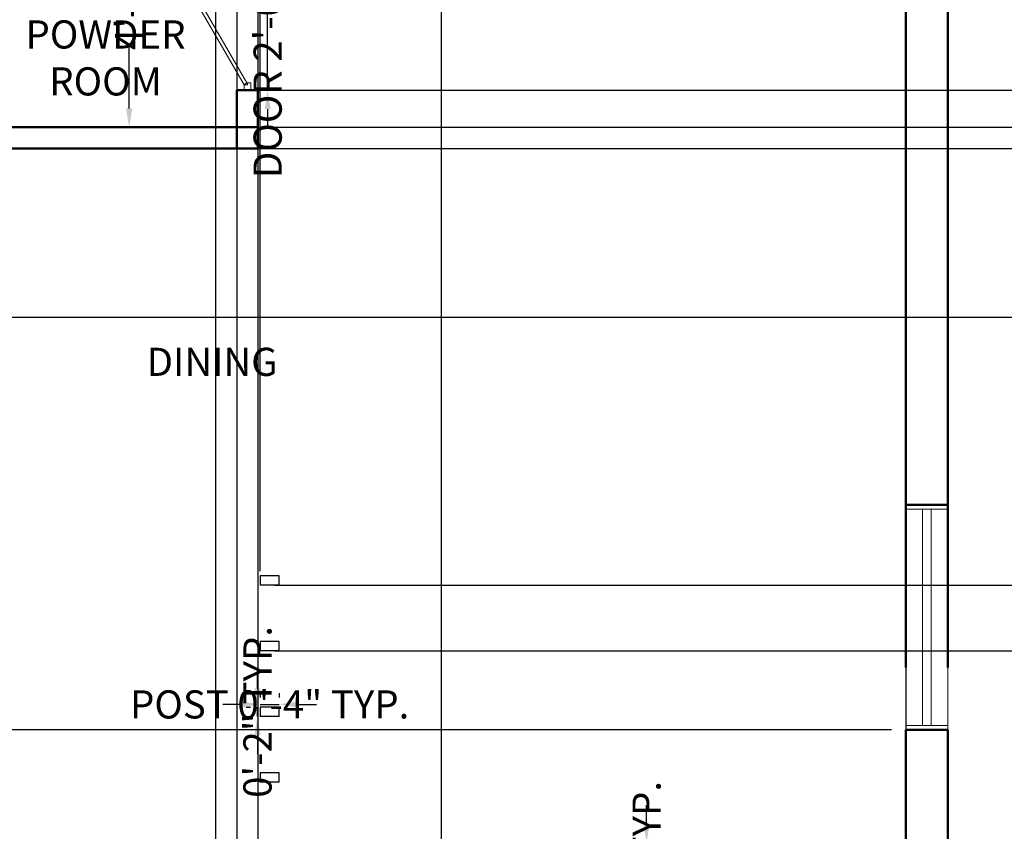
# Model space of a CAD drawing. Units: inches. Extents: x 6704 to 7574, y 11759 to 12617.
# Tile 5 of 8: x 7071 to 7281, y 12195 to 12368. Entities that reach past the tile are written whole.
import ezdxf

# ---------------------------------------------------------------- set-up
doc = ezdxf.new("R2010")
doc.units = ezdxf.units.IN
doc.header["$MEASUREMENT"] = 0
for name, color, linetype, lineweight in [('A-AREA-IDEN', 7, 'Continuous', 18), ('A-DOOR', 4, 'Continuous', 20), ('A-FLOR-SCRN', 7, 'Continuous', 25), ('WALL', 7, 'Continuous', 50), ('WINDOW', 2, 'Continuous', 20), ('YQ_DIM', 3, 'Continuous', 18)]:
    doc.layers.add(name, color=color, linetype=linetype, lineweight=lineweight)
doc.styles.get("Standard").update_dxf_attribs({"font": 'arial.ttf'})
doc.styles.add('YQ_DIM', font='SUPEROS.SHX', dxfattribs={"width": 0.8, "bigfont": 'HZDX.SHX'})
doc.dimstyles.new('yqi0', dxfattribs={"dimscale": 0, "dimtxt": 6, "dimasz": 4, "dimexe": 1.5, "dimexo": 3, "dimgap": 0.5, "dimtad": 0, "dimdsep": 46, "dimlunit": 4, "dimtxsty": 'Standard', "dimcen": 0, "dimclrd": 256, "dimclre": 256, "dimclrt": 7, "dimadec": 1, "dimazin": 2, "dimtfac": 1, "dimtix": 1, "dimtmove": 2, "dimatfit": 2, "dimfxl": 1, "dimtolj": 1, "dimtzin": 0, "dimarcsym": 0})

# ---------------------------------------------------------------- blocks, each defined once
blk = doc.blocks.new('*D5')
at = {"layer": 'Defpoints', "color": 0, "transparency": 16777216}
for p in [(7090.57, 12400.26), (7090.57, 12344.76), (7094.64, 12344.76)]:
    blk.add_point(p, dxfattribs=at)
at = {"layer": 'YQ_DIM', "color": 0, "lineweight": -2, "transparency": 16777216}
for p, q in [((7093.57, 12400.26), (7096.14, 12400.26)), ((7094.64, 12396.26), (7094.64, 12383.29)), ((7094.64, 12348.76), (7094.64, 12361.72)), ((7093.57, 12344.76), (7096.14, 12344.76))]:
    blk.add_line(p, q, dxfattribs=at)
at = {"layer": 'YQ_DIM', "color": 0, "transparency": 16777216}
for points in [[(7093.97, 12396.26), (7095.31, 12396.26), (7094.64, 12400.26)], [(7093.97, 12348.76), (7095.31, 12348.76), (7094.64, 12344.76)]]:
    blk.add_solid(points, dxfattribs=at)
at = {"layer": 'YQ_DIM', "color": 0, "transparency": 16777216, "insert": (7094.64, 12372.51), "char_height": 6, "attachment_point": 5, "rotation": 90}
blk.add_mtext('\\A1;4\'-7{\\H1x;\\S1/2;}"', dxfattribs=at)
blk = doc.blocks.new('WD_00_X1')
for p, q in [((-0.5, 0.5), (0.5, 0.5)), ((-0.48, 0.5), (-0.48, -0.5)), ((0.48, 0.5), (0.48, -0.5)), ((0.48, 0.1), (-0.48, 0.1)), ((0.48, -0.1), (-0.48, -0.1)), ((-0.5, -0.5), (0.5, -0.5))]:
    blk.add_line(p, q)
blk = doc.blocks.new('DR_CDR1')
for p, q in [((0.3294, 0.48), (-0.45, 0.03)), ((-0.435, 0.004), (0.3444, 0.454)), ((0.3294, 0.48), (0.3444, 0.454)), ((-0.45, 0.03), (-0.5, 0.03)), ((-0.435, 0.004), (-0.45, 0.03)), ((-0.45, 0.03), (-0.45, 0)), ((-0.45, 0), (-0.435, 0)), ((-0.435, 0), (-0.435, -0.03)), ((0.435, 0), (0.45, 0)), ((0.435, 0), (0.435, -0.03)), ((0.45, 0.03), (0.45, 0)), ((0.5, 0.03), (0.45, 0.03)), ((-0.435, -0.03), (-0.5, -0.03)), ((0.435, -0.03), (0.5, -0.03))]:
    blk.add_line(p, q)
blk.add_lwpolyline([(0.3444, 0.454, -0.121959), (0.45, 0.03)], format="xyb")
blk = doc.blocks.new('DIVIDER-POST-2X4')
for p, q in [((4, 2), (0, 2)), ((0, 2), (0, 0)), ((4, 0), (4, 2)), ((4, 0), (0, 0))]:
    blk.add_line(p, q)
blk = doc.blocks.new('*D26')
at = {"layer": 'Defpoints', "color": 0, "transparency": 16777216}
for p in [(7204.87, 12192.3), (7212.07, 12192.3), (7212.07, 12167.82)]:
    blk.add_point(p, dxfattribs=at)
at = {"layer": 'YQ_DIM', "lineweight": -2, "transparency": 16777216}
for p, q in [((7204.87, 12196.3), (7204.87, 12200.3)), ((7209.07, 12192.3), (7203.37, 12192.3)), ((7204.87, 12167.82), (7204.87, 12192.3)), ((7209.07, 12167.82), (7203.37, 12167.82)), ((7204.87, 12163.82), (7204.87, 12159.82))]:
    blk.add_line(p, q, dxfattribs=at)
at = {"layer": 'YQ_DIM', "transparency": 16777216}
for points in [[(7204.21, 12196.3), (7205.54, 12196.3), (7204.87, 12192.3)], [(7204.21, 12163.82), (7205.54, 12163.82), (7204.87, 12167.82)]]:
    blk.add_solid(points, dxfattribs=at)
at = {"layer": 'YQ_DIM', "color": 7, "transparency": 16777216, "insert": (7204.87, 12180.06), "char_height": 6, "attachment_point": 5, "rotation": 90}
blk.add_mtext('\\A1;2\'-0 1/2" TYP.', dxfattribs=at)
blk = doc.blocks.new('*D29')
at = {"layer": 'Defpoints', "color": 0, "transparency": 16777216}
for p in [(7120.54, 12376.63), (7124.14, 12376.63), (7120.54, 12352.63)]:
    blk.add_point(p, dxfattribs=at)
at = {"layer": 'YQ_DIM', "lineweight": -2, "transparency": 16777216}
for p, q in [((7124.14, 12380.63), (7124.14, 12384.63)), ((7123.54, 12376.63), (7125.64, 12376.63)), ((7124.14, 12352.63), (7124.14, 12376.63)), ((7123.54, 12352.63), (7125.64, 12352.63)), ((7124.14, 12348.63), (7124.14, 12344.63))]:
    blk.add_line(p, q, dxfattribs=at)
at = {"layer": 'YQ_DIM', "transparency": 16777216}
for points in [[(7123.48, 12380.63), (7124.81, 12380.63), (7124.14, 12376.63)], [(7123.48, 12348.63), (7124.81, 12348.63), (7124.14, 12352.63)]]:
    blk.add_solid(points, dxfattribs=at)
at = {"layer": 'YQ_DIM', "color": 7, "transparency": 16777216, "insert": (7124.14, 12364.63), "char_height": 6, "attachment_point": 5, "rotation": 90}
blk.add_mtext('\\A1;DOOR 2\'-0" TYP.', dxfattribs=at)
blk = doc.blocks.new('*D51')
at = {"layer": 'Defpoints', "color": 0, "transparency": 16777216}
for p in [(7122.57, 12221.15), (7126.57, 12221.75), (7126.57, 12221.15)]:
    blk.add_point(p, dxfattribs=at)
at = {"layer": 'YQ_DIM', "lineweight": -2, "transparency": 16777216}
for p, q in [((7122.57, 12224.15), (7122.57, 12223.25)), ((7126.57, 12224.15), (7126.57, 12223.25)), ((7118.57, 12221.75), (7114.57, 12221.75)), ((7122.57, 12221.75), (7126.57, 12221.75)), ((7130.57, 12221.75), (7134.57, 12221.75))]:
    blk.add_line(p, q, dxfattribs=at)
at = {"layer": 'YQ_DIM', "transparency": 16777216}
for points in [[(7118.57, 12222.42), (7118.57, 12221.09), (7122.57, 12221.75)], [(7130.57, 12222.42), (7130.57, 12221.09), (7126.57, 12221.75)]]:
    blk.add_solid(points, dxfattribs=at)
at = {"layer": 'YQ_DIM', "color": 7, "transparency": 16777216, "insert": (7124.57, 12221.75), "char_height": 6, "attachment_point": 5}
blk.add_mtext('\\A1;POST 0\'-4" TYP.', dxfattribs=at)
blk = doc.blocks.new('*D52')
at = {"layer": 'Defpoints', "color": 0, "transparency": 16777216}
for p in [(7121.97, 12221.15), (7122.57, 12221.15), (7122.57, 12219.15)]:
    blk.add_point(p, dxfattribs=at)
at = {"layer": 'YQ_DIM', "lineweight": -2, "transparency": 16777216}
for p, q in [((7121.97, 12225.15), (7121.97, 12229.15)), ((7119.57, 12221.15), (7120.47, 12221.15)), ((7121.97, 12219.15), (7121.97, 12221.15)), ((7119.57, 12219.15), (7120.47, 12219.15)), ((7121.97, 12215.15), (7121.97, 12211.15))]:
    blk.add_line(p, q, dxfattribs=at)
at = {"layer": 'YQ_DIM', "transparency": 16777216}
for points in [[(7121.31, 12225.15), (7122.64, 12225.15), (7121.97, 12221.15)], [(7121.31, 12215.15), (7122.64, 12215.15), (7121.97, 12219.15)]]:
    blk.add_solid(points, dxfattribs=at)
at = {"layer": 'YQ_DIM', "color": 7, "transparency": 16777216, "insert": (7121.97, 12220.15), "char_height": 6, "attachment_point": 5, "rotation": 90}
blk.add_mtext('\\A1;0\'-2" TYP.', dxfattribs=at)
blk = doc.blocks.new('*D60')
at = {"layer": 'Defpoints', "color": 0, "transparency": 16777216}
for p in [(7063.57, 12400.26), (7117.57, 12400.26), (7117.57, 11768.08)]:
    blk.add_point(p, dxfattribs=at)
at = {"layer": 'YQ_DIM', "lineweight": -2, "transparency": 16777216}
for p, q in [((7063.57, 12397.26), (7063.57, 11766.58)), ((7117.57, 12397.26), (7117.57, 11766.58)), ((7067.57, 11768.08), (7081.98, 11768.08)), ((7113.57, 11768.08), (7099.17, 11768.08))]:
    blk.add_line(p, q, dxfattribs=at)
at = {"layer": 'YQ_DIM', "transparency": 16777216}
for points in [[(7067.57, 11768.74), (7067.57, 11767.41), (7063.57, 11768.08)], [(7113.57, 11768.74), (7113.57, 11767.41), (7117.57, 11768.08)]]:
    blk.add_solid(points, dxfattribs=at)
at = {"layer": 'YQ_DIM', "color": 7, "transparency": 16777216, "insert": (7090.57, 11768.08), "char_height": 6, "attachment_point": 5}
blk.add_mtext('\\A1;4\'-6"', dxfattribs=at)
blk = doc.blocks.new('*D62')
at = {"layer": 'Defpoints', "color": 0, "transparency": 16777216}
for p in [(7260.07, 12419.43), (7122.07, 12340.26), (7260.07, 11768.08)]:
    blk.add_point(p, dxfattribs=at)
at = {"layer": 'YQ_DIM', "lineweight": -2, "transparency": 16777216}
for p, q in [((7260.07, 12416.43), (7260.07, 11766.58)), ((7122.07, 12337.26), (7122.07, 11766.58)), ((7126.07, 11768.08), (7180.55, 11768.08)), ((7256.07, 11768.08), (7201.6, 11768.08))]:
    blk.add_line(p, q, dxfattribs=at)
at = {"layer": 'YQ_DIM', "transparency": 16777216}
for points in [[(7126.07, 11768.74), (7126.07, 11767.41), (7122.07, 11768.08)], [(7256.07, 11768.74), (7256.07, 11767.41), (7260.07, 11768.08)]]:
    blk.add_solid(points, dxfattribs=at)
at = {"layer": 'YQ_DIM', "color": 7, "transparency": 16777216, "insert": (7191.07, 11768.08), "char_height": 6, "attachment_point": 5}
blk.add_mtext('\\A1;11\'-6"', dxfattribs=at)
blk = doc.blocks.new('*D63')
at = {"layer": 'Defpoints', "color": 0, "transparency": 16777216}
for p in [(7269.07, 12511.26), (7565.25, 12511.26), (7269.07, 12164.76)]:
    blk.add_point(p, dxfattribs=at)
at = {"layer": 'YQ_DIM', "lineweight": -2, "transparency": 16777216}
for p, q in [((7272.07, 12511.26), (7566.75, 12511.26)), ((7565.25, 12507.26), (7565.25, 12358.19)), ((7565.25, 12168.76), (7565.25, 12317.83)), ((7272.07, 12164.76), (7566.75, 12164.76))]:
    blk.add_line(p, q, dxfattribs=at)
at = {"layer": 'YQ_DIM', "transparency": 16777216}
for points in [[(7564.58, 12507.26), (7565.91, 12507.26), (7565.25, 12511.26)], [(7564.58, 12168.76), (7565.91, 12168.76), (7565.25, 12164.76)]]:
    blk.add_solid(points, dxfattribs=at)
at = {"layer": 'YQ_DIM', "color": 7, "transparency": 16777216, "insert": (7565.25, 12338.01), "char_height": 6, "attachment_point": 5, "rotation": 90}
blk.add_mtext('\\A1;28\'-10 1/2"', dxfattribs=at)
blk = doc.blocks.new('*D65')
at = {"layer": 'Defpoints', "color": 0, "transparency": 16777216}
for p in [(7113.07, 12590.81), (7062.07, 12121.26), (7113.07, 12121.26)]:
    blk.add_point(p, dxfattribs=at)
at = {"layer": 'YQ_DIM', "lineweight": -2, "transparency": 16777216}
for p, q in [((7062.07, 12124.26), (7062.07, 12592.31)), ((7113.07, 12124.26), (7113.07, 12592.31)), ((7066.07, 12590.81), (7078.98, 12590.81)), ((7109.07, 12590.81), (7096.17, 12590.81))]:
    blk.add_line(p, q, dxfattribs=at)
at = {"layer": 'YQ_DIM', "transparency": 16777216}
for points in [[(7066.07, 12591.47), (7066.07, 12590.14), (7062.07, 12590.81)], [(7109.07, 12591.47), (7109.07, 12590.14), (7113.07, 12590.81)]]:
    blk.add_solid(points, dxfattribs=at)
at = {"layer": 'YQ_DIM', "color": 7, "transparency": 16777216, "insert": (7087.57, 12590.81), "char_height": 6, "attachment_point": 5}
blk.add_mtext('\\A1;4\'-3"', dxfattribs=at)
blk = doc.blocks.new('*D68')
at = {"layer": 'Defpoints', "color": 0, "transparency": 16777216}
for p in [(6927.07, 12340.26), (7565.25, 12340.26), (6927.07, 12304.26)]:
    blk.add_point(p, dxfattribs=at)
at = {"layer": 'YQ_DIM', "lineweight": -2, "transparency": 16777216}
for p, q in [((6930.07, 12340.26), (7566.75, 12340.26)), ((7565.25, 12336.26), (7565.25, 12330.73)), ((7565.25, 12308.26), (7565.25, 12313.78)), ((6930.07, 12304.26), (7566.75, 12304.26))]:
    blk.add_line(p, q, dxfattribs=at)
at = {"layer": 'YQ_DIM', "transparency": 16777216}
for points in [[(7564.58, 12336.26), (7565.91, 12336.26), (7565.25, 12340.26)], [(7564.58, 12308.26), (7565.91, 12308.26), (7565.25, 12304.26)]]:
    blk.add_solid(points, dxfattribs=at)
at = {"layer": 'YQ_DIM', "color": 7, "transparency": 16777216, "insert": (7565.25, 12322.26), "char_height": 6, "attachment_point": 5, "rotation": 90}
blk.add_mtext('\\A1;3\'-0"', dxfattribs=at)
blk = doc.blocks.new('*D69')
at = {"layer": 'Defpoints', "color": 0, "transparency": 16777216}
for p in [(7122.57, 12247.15), (7122.57, 12233.15), (7565.25, 12233.15)]:
    blk.add_point(p, dxfattribs=at)
at = {"layer": 'YQ_DIM', "lineweight": -2, "transparency": 16777216}
for p, q in [((7565.25, 12251.15), (7565.25, 12255.15)), ((7125.57, 12247.15), (7566.75, 12247.15)), ((7565.25, 12247.15), (7565.25, 12233.15)), ((7125.57, 12233.15), (7566.75, 12233.15)), ((7565.25, 12229.15), (7565.25, 12225.15))]:
    blk.add_line(p, q, dxfattribs=at)
at = {"layer": 'YQ_DIM', "transparency": 16777216}
for points in [[(7564.58, 12251.15), (7565.91, 12251.15), (7565.25, 12247.15)], [(7564.58, 12229.15), (7565.91, 12229.15), (7565.25, 12233.15)]]:
    blk.add_solid(points, dxfattribs=at)
at = {"layer": 'YQ_DIM', "color": 7, "transparency": 16777216, "insert": (7565.25, 12240.15), "char_height": 6, "attachment_point": 5, "rotation": 90}
blk.add_mtext('\\A1;1\'-2"', dxfattribs=at)
blk = doc.blocks.new('*D77')
at = {"layer": 'Defpoints', "color": 0, "transparency": 16777216}
for p in [(7260.07, 12216.3), (6712.97, 12173.76), (7260.07, 12173.76)]:
    blk.add_point(p, dxfattribs=at)
at = {"layer": 'YQ_DIM', "lineweight": -2, "transparency": 16777216}
for p, q in [((7257.07, 12216.3), (6711.47, 12216.3)), ((6712.97, 12212.3), (6712.97, 12210.49)), ((6712.97, 12177.76), (6712.97, 12179.57)), ((7257.07, 12173.76), (6711.47, 12173.76))]:
    blk.add_line(p, q, dxfattribs=at)
at = {"layer": 'YQ_DIM', "transparency": 16777216}
for points in [[(6712.3, 12212.3), (6713.64, 12212.3), (6712.97, 12216.3)], [(6712.3, 12177.76), (6713.64, 12177.76), (6712.97, 12173.76)]]:
    blk.add_solid(points, dxfattribs=at)
at = {"layer": 'YQ_DIM', "color": 7, "transparency": 16777216, "insert": (6712.97, 12195.03), "char_height": 6, "attachment_point": 5, "rotation": 90}
blk.add_mtext('\\A1;3\'-6 1/2"', dxfattribs=at)
blk = doc.blocks.new('*D82')
at = {"layer": 'Defpoints', "color": 0, "transparency": 16777216}
for p in [(7117.57, 12352.63), (7565.25, 12352.63), (7122.07, 12344.76)]:
    blk.add_point(p, dxfattribs=at)
at = {"layer": 'YQ_DIM', "lineweight": -2, "transparency": 16777216}
for p, q in [((7565.25, 12356.63), (7565.25, 12360.63)), ((7120.57, 12352.63), (7566.75, 12352.63)), ((7565.25, 12344.76), (7565.25, 12352.63)), ((7125.07, 12344.76), (7566.75, 12344.76)), ((7565.25, 12340.76), (7565.25, 12336.76))]:
    blk.add_line(p, q, dxfattribs=at)
at = {"layer": 'YQ_DIM', "transparency": 16777216}
for points in [[(7564.58, 12356.63), (7565.91, 12356.63), (7565.25, 12352.63)], [(7564.58, 12340.76), (7565.91, 12340.76), (7565.25, 12344.76)]]:
    blk.add_solid(points, dxfattribs=at)
at = {"layer": 'YQ_DIM', "color": 7, "transparency": 16777216, "insert": (7565.25, 12348.69), "char_height": 6, "attachment_point": 5, "rotation": 90}
blk.add_mtext('\\A1;0\'-8"', dxfattribs=at)
blk = doc.blocks.new('*D85')
at = {"layer": 'Defpoints', "color": 0, "transparency": 16777216}
for p in [(7122.07, 12502.26), (7161.07, 12502.26), (7161.07, 11768.08)]:
    blk.add_point(p, dxfattribs=at)
at = {"layer": 'YQ_DIM', "lineweight": -2, "transparency": 16777216}
for p, q in [((7122.07, 12499.26), (7122.07, 11766.58)), ((7161.07, 12499.26), (7161.07, 11766.58)), ((7126.07, 11768.08), (7133.1, 11768.08)), ((7157.07, 11768.08), (7150.05, 11768.08))]:
    blk.add_line(p, q, dxfattribs=at)
at = {"layer": 'YQ_DIM', "transparency": 16777216}
for points in [[(7126.07, 11768.74), (7126.07, 11767.41), (7122.07, 11768.08)], [(7157.07, 11768.74), (7157.07, 11767.41), (7161.07, 11768.08)]]:
    blk.add_solid(points, dxfattribs=at)
at = {"layer": 'YQ_DIM', "color": 7, "transparency": 16777216, "insert": (7141.57, 11768.08), "char_height": 6, "attachment_point": 5}
blk.add_mtext('\\A1;3\'-3"', dxfattribs=at)
blk = doc.blocks.new('*D88')
at = {"layer": 'Defpoints', "color": 0, "transparency": 16777216}
for p in [(7260.07, 12590.81), (7260.07, 12264.3), (7122.57, 12247.15)]:
    blk.add_point(p, dxfattribs=at)
at = {"layer": 'YQ_DIM', "lineweight": -2, "transparency": 16777216}
for p, q in [((7122.57, 12250.15), (7122.57, 12592.31)), ((7260.07, 12267.3), (7260.07, 12592.31)), ((7126.57, 12590.81), (7173.81, 12590.81)), ((7256.07, 12590.81), (7208.84, 12590.81))]:
    blk.add_line(p, q, dxfattribs=at)
at = {"layer": 'YQ_DIM', "transparency": 16777216}
for points in [[(7126.57, 12591.47), (7126.57, 12590.14), (7122.57, 12590.81)], [(7256.07, 12591.47), (7256.07, 12590.14), (7260.07, 12590.81)]]:
    blk.add_solid(points, dxfattribs=at)
at = {"layer": 'YQ_DIM', "color": 7, "transparency": 16777216, "insert": (7191.32, 12590.81), "char_height": 6, "attachment_point": 5}
blk.add_mtext('\\A1;11\'-5 1/2"', dxfattribs=at)

msp = doc.modelspace()

# ---------------------------------------------------------------- linework, layer by layer
at = {"layer": 'WALL'}
for p, q in [((7260.073, 12229.631), (7260.073, 12446.383)), ((7269.073, 12229.631), (7269.073, 12446.383)), ((7117.573, 12340.257), (7117.573, 12352.631)), ((7117.573, 12352.631), (7122.073, 12352.631)), ((7122.073, 12340.257), (7122.073, 12352.631)), ((7051.198, 12344.757), (7122.073, 12344.757)), ((7051.198, 12340.257), (7122.073, 12340.257)), ((7260.073, 12264.302), (7269.073, 12264.302)), ((7260.073, 12173.757), (7260.073, 12216.302)), ((7260.073, 12216.302), (7269.073, 12216.302)), ((7269.073, 12164.757), (7269.073, 12216.302))]:
    msp.add_line(p, q, dxfattribs=at)

# ---------------------------------------------------------------- block references
at = {"layer": 'A-DOOR', "xscale": 24, "yscale": 24, "zscale": 24, "rotation": 90}
msp.add_blockref('DR_CDR1', (7119.823, 12364.631), dxfattribs=at)
at = {"layer": 'A-FLOR-SCRN'}
for p in [(7122.573, 12247.154), (7122.573, 12233.154), (7122.573, 12219.154), (7122.573, 12205.154)]:
    msp.add_blockref('DIVIDER-POST-2X4', p, dxfattribs=at)
at = {"layer": 'WINDOW', "xscale": 48, "yscale": 9, "zscale": 48, "rotation": 90}
msp.add_blockref('WD_00_X1', (7264.573, 12240.302), dxfattribs=at)

# ---------------------------------------------------------------- texts
at = {"layer": 'A-AREA-IDEN', "char_height": 13.77953, "width": 31.54746, "attachment_point": 1, "style": 'YQ_DIM'}
for s, insert in [('\\pxqc;{\\H0.43543x;POWDER ROOM}', (7073.83, 12367.53)), ('\\pxqc;{\\H0.43543x;DINING}', (7096.541, 12297.763))]:
    msp.add_mtext(s, dxfattribs=dict(at, insert=insert))

# ---------------------------------------------------------------- dimensions: what is measured, and where the dimension line sits
at = {"layer": 'YQ_DIM'}
for base, p1, p2, picture, middle in [((7260.073, 12590.807), (7122.573, 12247.154), (7260.073, 12264.302), '*D88', (7191.323, 12590.807)), ((7113.073, 12590.807), (7062.073, 12121.257), (7113.073, 12121.257), '*D65', (7087.573, 12590.807)), ((7161.073, 11768.077), (7122.073, 12502.257), (7161.073, 12502.257), '*D85', (7141.573, 11768.077)), ((7260.073, 11768.077), (7122.073, 12340.257), (7260.073, 12419.428), '*D62', (7191.073, 11768.077)), ((7117.573, 11768.077), (7063.573, 12400.257), (7117.573, 12400.257), '*D60', (7090.573, 11768.077))]:
    dim = msp.add_linear_dim(base=base, p1=p1, p2=p2, dimstyle='yqi0', override={"dimscale": 1, "dimdec": 1, "dimzin": 1, "dimfrac": 2}, dxfattribs=at)
    dim.commit()
    dim.dimension.update_dxf_attribs({"geometry": picture, "text_midpoint": middle})
for base, p1, p2, picture, middle in [((7565.248, 12511.257), (7269.073, 12164.757), (7269.073, 12511.257), '*D63', (7565.248, 12338.007)), ((7565.248, 12352.631), (7122.073, 12344.757), (7117.573, 12352.631), '*D82', (7565.248, 12348.694)), ((7565.248, 12340.257), (6927.073, 12304.257), (6927.073, 12340.257), '*D68', (7565.248, 12322.257)), ((7565.248, 12233.154), (7122.573, 12247.154), (7122.573, 12233.154), '*D69', (7565.248, 12240.154)), ((6712.97, 12173.757), (7260.073, 12216.302), (7260.073, 12173.757), '*D77', (6712.97, 12195.029))]:
    dim = msp.add_linear_dim(base=base, p1=p1, p2=p2, angle=90, dimstyle='yqi0', override={"dimscale": 1, "dimdec": 1, "dimzin": 1, "dimfrac": 2}, dxfattribs=at)
    dim.commit()
    dim.dimension.update_dxf_attribs({"geometry": picture, "text_midpoint": middle})
dim = msp.add_aligned_dim(p1=(7090.573, 12400.257), p2=(7090.573, 12344.757), distance=4.067, dimstyle='yqi0', override={"dimscale": 1, "dimclrd": 0, "dimclre": 0, "dimclrt": 0}, dxfattribs=at)
dim.commit()
dim.dimension.update_dxf_attribs({"geometry": '*D5', "text_midpoint": (7094.64, 12372.507)})
for base, p1, p2, text, picture, middle in [((7124.143, 12376.631), (7120.543, 12352.631), (7120.543, 12376.631), 'DOOR <> TYP.', '*D29', (7124.143, 12364.631)), ((7121.973, 12221.154), (7122.573, 12219.154), (7122.573, 12221.154), '<> TYP.', '*D52', (7121.973, 12220.154)), ((7204.873, 12192.297), (7212.073, 12167.817), (7212.073, 12192.297), '<> TYP.', '*D26', (7204.873, 12180.057))]:
    dim = msp.add_linear_dim(base=base, p1=p1, p2=p2, angle=90, text=text, dimstyle='yqi0', override={"dimscale": 1, "dimdec": 1, "dimzin": 1, "dimfrac": 2}, dxfattribs=at)
    dim.commit()
    dim.dimension.update_dxf_attribs({"geometry": picture, "text_midpoint": middle})
dim = msp.add_linear_dim(base=(7126.573, 12221.754), p1=(7122.573, 12221.154), p2=(7126.573, 12221.154), text='POST <> TYP.', dimstyle='yqi0', override={"dimscale": 1, "dimdec": 1, "dimzin": 1, "dimfrac": 2}, dxfattribs=at)
dim.commit()
dim.dimension.update_dxf_attribs({"geometry": '*D51', "text_midpoint": (7124.573, 12221.754)})

doc.saveas('drawing.dxf')
